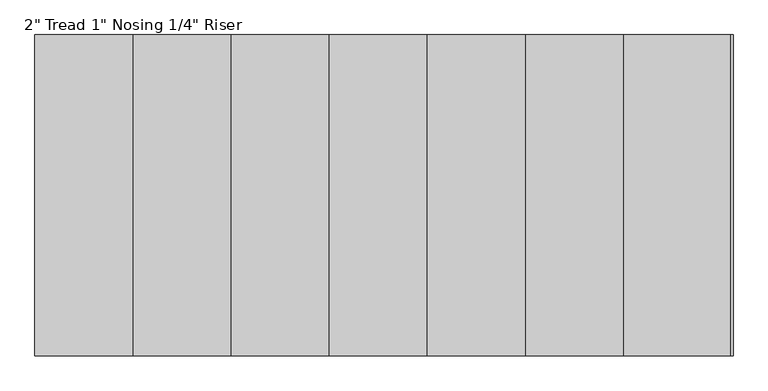
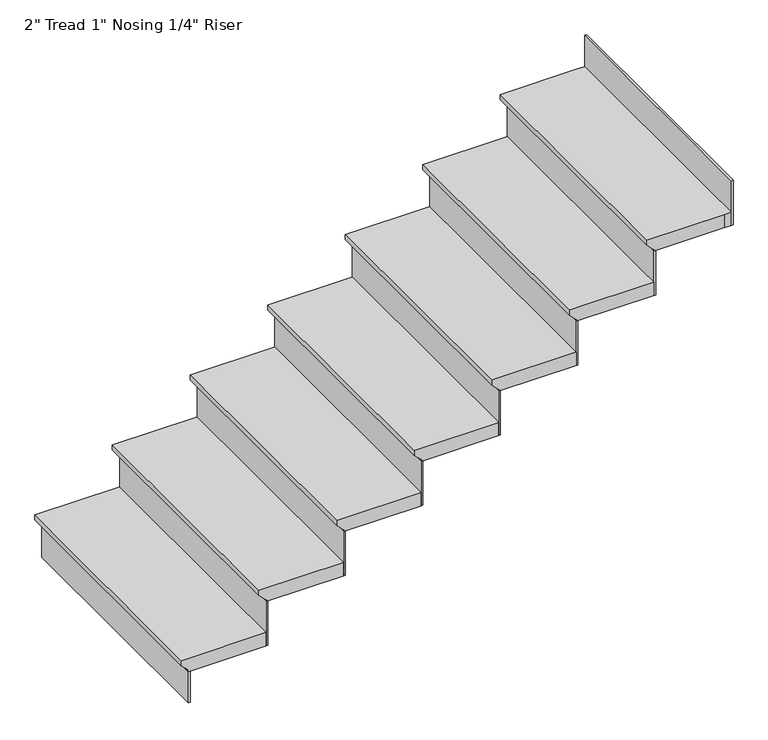
"""IFC4 building model written with IfcOpenShell, lengths in millimetres: stair flight geometry."""

from ifc_helpers import new_model, si_unit, origin, place, context, project, spatial, faceted_brep, source, transform, mapped, element, save


def stair_flight_5027378a(model_context):
    return source(origin(), model_context, "Body", "Brep", [
        faceted_brep([(-1404.564062, 2339.7857363, 302.6833333), (-1404.564062, 2339.7857363, 321.7333333), (-1404.564062, 3254.1857363, 321.7333333), (-1404.564062, 3254.1857363, 302.6833333), (-1379.164062, 2339.7857363, 277.2833333), (-1379.164062, 3254.1857363, 277.2833333), (-1099.764062, 2339.7857363, 321.7333333), (-1099.764062, 3254.1857363, 321.7333333), (-1379.164062, 3254.1857363, 270.9333333), (-1099.764062, 3254.1857363, 270.9333333), (-1099.764062, 2339.7857363, 270.9333333), (-1379.164062, 2339.7857363, 270.9333333)], [[[0, 1, 2, 3]], [[4, 0, 3, 5]], [[2, 1, 6, 7]], [[8, 9, 10, 11]], [[2, 7, 9, 8, 5, 3]], [[8, 11, 4, 5]], [[6, 1, 0, 4, 11, 10]], [[7, 6, 10, 9]]]),
        faceted_brep([(-1379.164062, 2339.7857363, 270.9333333), (-1379.164062, 2339.7857363, 152.4), (-1372.814062, 2339.7857363, 152.4), (-1372.814062, 2339.7857363, 270.9333333), (-1379.164062, 3254.1857363, 270.9333333), (-1372.814062, 3254.1857363, 270.9333333), (-1372.814062, 3254.1857363, 152.4), (-1379.164062, 3254.1857363, 152.4)], [[[0, 1, 2, 3]], [[4, 5, 6, 7]], [[1, 0, 4, 7]], [[2, 1, 7, 6]], [[3, 2, 6, 5]], [[0, 3, 5, 4]]]),
        faceted_brep([(-1099.764062, 2339.7857363, 440.2666667), (-1099.764062, 2339.7857363, 270.9333333), (-1093.414062, 2339.7857363, 270.9333333), (-1093.414062, 2339.7857363, 440.2666667), (-1099.764062, 3254.1857363, 440.2666667), (-1093.414062, 3254.1857363, 440.2666667), (-1093.414062, 3254.1857363, 270.9333333), (-1099.764062, 3254.1857363, 270.9333333)], [[[0, 1, 2, 3]], [[4, 5, 6, 7]], [[1, 0, 4, 7]], [[2, 1, 7, 6]], [[3, 2, 6, 5]], [[0, 3, 5, 4]]]),
        faceted_brep([(-1125.164062, 3254.1857363, 491.0666667), (-1125.164062, 2339.7857363, 491.0666667), (-820.364062, 2339.7857363, 491.0666667), (-820.364062, 3254.1857363, 491.0666667), (-1099.764062, 3254.1857363, 440.2666667), (-820.364062, 3254.1857363, 440.2666667), (-820.364062, 2339.7857363, 440.2666667), (-1099.764062, 2339.7857363, 440.2666667), (-1099.764062, 3254.1857363, 446.6166667), (-1125.164062, 3254.1857363, 472.0166667), (-1099.764062, 2339.7857363, 446.6166667), (-1125.164062, 2339.7857363, 472.0166667)], [[[0, 1, 2, 3]], [[4, 5, 6, 7]], [[0, 3, 5, 4, 8, 9]], [[4, 7, 10, 8]], [[2, 1, 11, 10, 7, 6]], [[3, 2, 6, 5]], [[11, 1, 0, 9]], [[10, 11, 9, 8]]]),
        faceted_brep([(-820.364062, 2339.7857363, 609.6), (-820.364062, 2339.7857363, 440.2666667), (-814.014062, 2339.7857363, 440.2666667), (-814.014062, 2339.7857363, 609.6), (-820.364062, 3254.1857363, 609.6), (-814.014062, 3254.1857363, 609.6), (-814.014062, 3254.1857363, 440.2666667), (-820.364062, 3254.1857363, 440.2666667)], [[[0, 1, 2, 3]], [[4, 5, 6, 7]], [[1, 0, 4, 7]], [[2, 1, 7, 6]], [[3, 2, 6, 5]], [[0, 3, 5, 4]]]),
        faceted_brep([(-845.764062, 3254.1857363, 660.4), (-845.764062, 2339.7857363, 660.4), (-540.964062, 2339.7857363, 660.4), (-540.964062, 3254.1857363, 660.4), (-820.364062, 3254.1857363, 609.6), (-540.964062, 3254.1857363, 609.6), (-540.964062, 2339.7857363, 609.6), (-820.364062, 2339.7857363, 609.6), (-820.364062, 3254.1857363, 615.95), (-845.764062, 3254.1857363, 641.35), (-820.364062, 2339.7857363, 615.95), (-845.764062, 2339.7857363, 641.35)], [[[0, 1, 2, 3]], [[4, 5, 6, 7]], [[0, 3, 5, 4, 8, 9]], [[4, 7, 10, 8]], [[2, 1, 11, 10, 7, 6]], [[3, 2, 6, 5]], [[11, 1, 0, 9]], [[10, 11, 9, 8]]]),
        faceted_brep([(-540.964062, 2339.7857363, 778.9333333), (-540.964062, 2339.7857363, 609.6), (-534.614062, 2339.7857363, 609.6), (-534.614062, 2339.7857363, 778.9333333), (-540.964062, 3254.1857363, 778.9333333), (-534.614062, 3254.1857363, 778.9333333), (-534.614062, 3254.1857363, 609.6), (-540.964062, 3254.1857363, 609.6)], [[[0, 1, 2, 3]], [[4, 5, 6, 7]], [[1, 0, 4, 7]], [[2, 1, 7, 6]], [[3, 2, 6, 5]], [[0, 3, 5, 4]]]),
        faceted_brep([(-566.364062, 3254.1857363, 829.7333333), (-566.364062, 2339.7857363, 829.7333333), (-261.564062, 2339.7857363, 829.7333333), (-261.564062, 3254.1857363, 829.7333333), (-540.964062, 3254.1857363, 778.9333333), (-261.564062, 3254.1857363, 778.9333333), (-261.564062, 2339.7857363, 778.9333333), (-540.964062, 2339.7857363, 778.9333333), (-540.964062, 3254.1857363, 785.2833333), (-566.364062, 3254.1857363, 810.6833333), (-540.964062, 2339.7857363, 785.2833333), (-566.364062, 2339.7857363, 810.6833333)], [[[0, 1, 2, 3]], [[4, 5, 6, 7]], [[0, 3, 5, 4, 8, 9]], [[4, 7, 10, 8]], [[2, 1, 11, 10, 7, 6]], [[3, 2, 6, 5]], [[11, 1, 0, 9]], [[10, 11, 9, 8]]]),
        faceted_brep([(-261.564062, 2339.7857363, 948.2666667), (-261.564062, 2339.7857363, 778.9333333), (-255.214062, 2339.7857363, 778.9333333), (-255.214062, 2339.7857363, 948.2666667), (-261.564062, 3254.1857363, 948.2666667), (-255.214062, 3254.1857363, 948.2666667), (-255.214062, 3254.1857363, 778.9333333), (-261.564062, 3254.1857363, 778.9333333)], [[[0, 1, 2, 3]], [[4, 5, 6, 7]], [[1, 0, 4, 7]], [[2, 1, 7, 6]], [[3, 2, 6, 5]], [[0, 3, 5, 4]]]),
        faceted_brep([(-286.964062, 3254.1857363, 999.0666667), (-286.964062, 2339.7857363, 999.0666667), (17.835938, 2339.7857363, 999.0666667), (17.835938, 3254.1857363, 999.0666667), (-261.564062, 3254.1857363, 948.2666667), (17.835938, 3254.1857363, 948.2666667), (17.835938, 2339.7857363, 948.2666667), (-261.564062, 2339.7857363, 948.2666667), (-261.564062, 3254.1857363, 954.6166667), (-286.964062, 3254.1857363, 980.0166667), (-261.564062, 2339.7857363, 954.6166667), (-286.964062, 2339.7857363, 980.0166667)], [[[0, 1, 2, 3]], [[4, 5, 6, 7]], [[0, 3, 5, 4, 8, 9]], [[4, 7, 10, 8]], [[2, 1, 11, 10, 7, 6]], [[3, 2, 6, 5]], [[11, 1, 0, 9]], [[10, 11, 9, 8]]]),
        faceted_brep([(17.835938, 2339.7857363, 1117.6), (17.835938, 2339.7857363, 948.2666667), (24.185938, 2339.7857363, 948.2666667), (24.185938, 2339.7857363, 1117.6), (17.835938, 3254.1857363, 1117.6), (24.185938, 3254.1857363, 1117.6), (24.185938, 3254.1857363, 948.2666667), (17.835938, 3254.1857363, 948.2666667)], [[[0, 1, 2, 3]], [[4, 5, 6, 7]], [[1, 0, 4, 7]], [[2, 1, 7, 6]], [[3, 2, 6, 5]], [[0, 3, 5, 4]]]),
        faceted_brep([(-7.564062, 3254.1857363, 1168.4), (-7.564062, 2339.7857363, 1168.4), (297.235938, 2339.7857363, 1168.4), (297.235938, 3254.1857363, 1168.4), (17.835938, 3254.1857363, 1117.6), (297.235938, 3254.1857363, 1117.6), (297.235938, 2339.7857363, 1117.6), (17.835938, 2339.7857363, 1117.6), (17.835938, 3254.1857363, 1123.95), (-7.564062, 3254.1857363, 1149.35), (17.835938, 2339.7857363, 1123.95), (-7.564062, 2339.7857363, 1149.35)], [[[0, 1, 2, 3]], [[4, 5, 6, 7]], [[0, 3, 5, 4, 8, 9]], [[4, 7, 10, 8]], [[2, 1, 11, 10, 7, 6]], [[3, 2, 6, 5]], [[11, 1, 0, 9]], [[10, 11, 9, 8]]]),
        faceted_brep([(576.635938, 2339.7857363, 1456.2666667), (576.635938, 2339.7857363, 1286.9333333), (582.985938, 2339.7857363, 1286.9333333), (582.985938, 2339.7857363, 1456.2666667), (576.635938, 3254.1857363, 1456.2666667), (582.985938, 3254.1857363, 1456.2666667), (582.985938, 3254.1857363, 1286.9333333), (576.635938, 3254.1857363, 1286.9333333)], [[[0, 1, 2, 3]], [[4, 5, 6, 7]], [[1, 0, 4, 7]], [[2, 1, 7, 6]], [[3, 2, 6, 5]], [[0, 3, 5, 4]]]),
        faceted_brep([(297.235938, 2339.7857363, 1286.9333333), (297.235938, 2339.7857363, 1117.6), (303.585938, 2339.7857363, 1117.6), (303.585938, 2339.7857363, 1286.9333333), (297.235938, 3254.1857363, 1286.9333333), (303.585938, 3254.1857363, 1286.9333333), (303.585938, 3254.1857363, 1117.6), (297.235938, 3254.1857363, 1117.6)], [[[0, 1, 2, 3]], [[4, 5, 6, 7]], [[1, 0, 4, 7]], [[2, 1, 7, 6]], [[3, 2, 6, 5]], [[0, 3, 5, 4]]]),
        faceted_brep([(576.635938, 3254.1857363, 1337.7333333), (551.235938, 3254.1857363, 1337.7333333), (271.835938, 3254.1857363, 1337.7333333), (271.835938, 2339.7857363, 1337.7333333), (551.235938, 2339.7857363, 1337.7333333), (576.635938, 2339.7857363, 1337.7333333), (551.235938, 3254.1857363, 1286.9333333), (576.635938, 3254.1857363, 1286.9333333), (576.635938, 2339.7857363, 1286.9333333), (551.235938, 2339.7857363, 1286.9333333), (297.235938, 2339.7857363, 1286.9333333), (297.235938, 3254.1857363, 1286.9333333), (297.235938, 3254.1857363, 1293.2833333), (271.835938, 3254.1857363, 1318.6833333), (297.235938, 2339.7857363, 1293.2833333), (271.835938, 2339.7857363, 1318.6833333)], [[[0, 1, 2, 3, 4, 5]], [[6, 7, 8, 9, 10, 11]], [[1, 0, 7, 6]], [[2, 1, 6, 11, 12, 13]], [[11, 10, 14, 12]], [[4, 3, 15, 14, 10, 9]], [[5, 4, 9, 8]], [[0, 5, 8, 7]], [[15, 3, 2, 13]], [[14, 15, 13, 12]]]),
    ])


if __name__ == "__main__":
    model = new_model("IFC4")
    model_context = context("Model", 3, world=origin())
    ifc_project = project(units=[si_unit("LENGTHUNIT", "METRE", prefix="MILLI")], contexts=[model_context])
    site = spatial("IfcSite", under=ifc_project)
    building = spatial("IfcBuilding", under=site)
    placement = place(None, origin())
    stair_flight_shape = stair_flight_5027378a(model_context)
    element("IfcStairFlight", 1, ObjectType="2\" Tread 1\" Nosing 1/4\" Riser", at=placement, inside=building, context=model_context, shape_type="MappedRepresentation", body=[
        mapped(stair_flight_shape, transform((0.0, 0.0, 0.0), x_axis=(1.0, 0.0, 0.0), y_axis=(0.0, 1.0, 0.0), z_axis=(0.0, 0.0, 1.0))),
    ])
    save(model, "model.ifc")

# Revit data of these elements
# Element 1 (IfcStairFlight, "2\" Tread 1\" Nosing 1/4\" Riser")
#   Materials on its faces: "BURGUNDY COLOUR"
# Materials
#   "BURGUNDY COLOUR": class "Generic", colour RGB 120 120 120, transparency 0, Cost = 0
